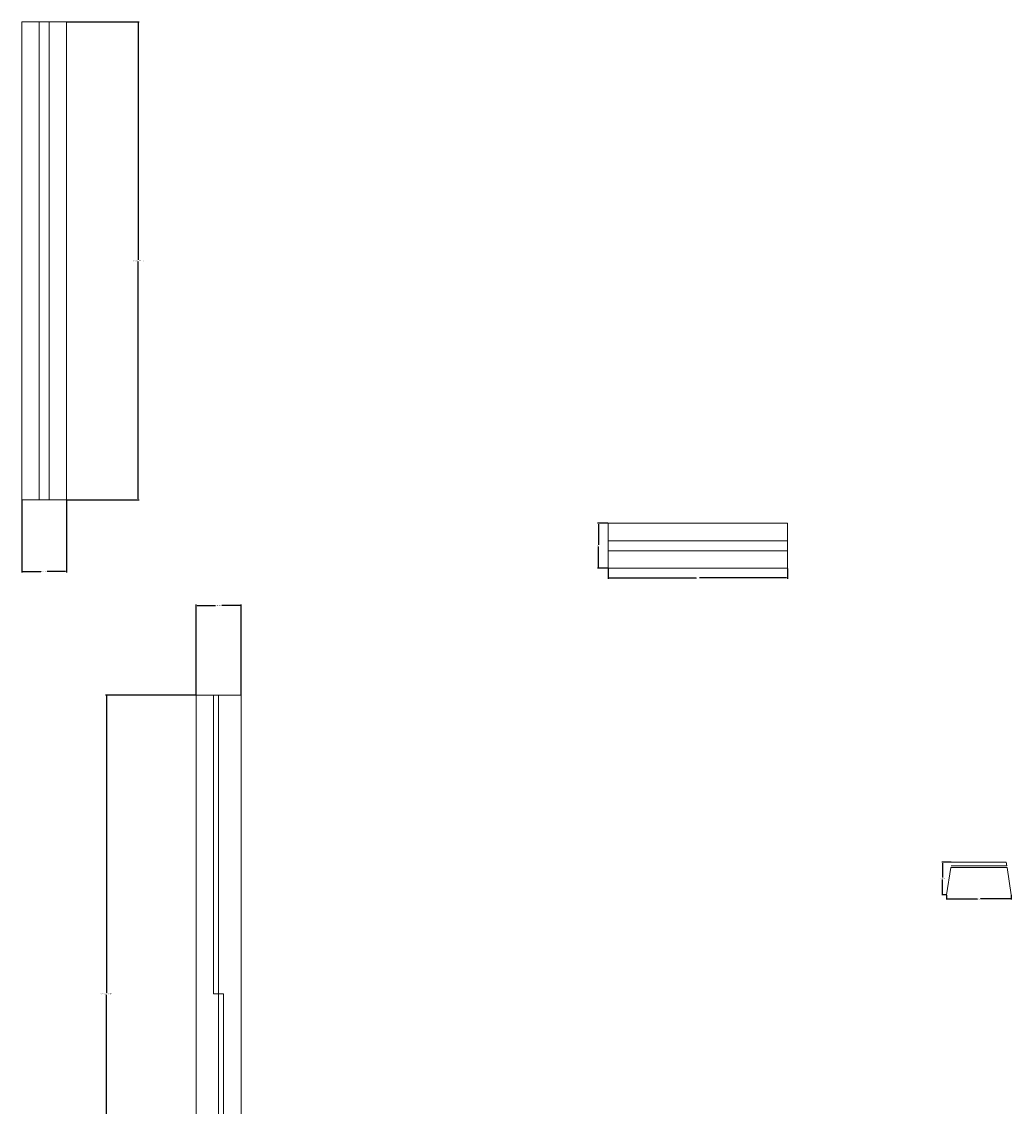
# Model space of a CAD drawing. Units: inches. Extents: x 226 to 1155, y 22 to 494.
# Tile 7 of 7: x 952 to 1150, y 276 to 494. Entities that reach past the tile are written whole.
import ezdxf

# ---------------------------------------------------------------- set-up
doc = ezdxf.new("R2010")
doc.units = ezdxf.units.IN
doc.header["$MEASUREMENT"] = 0
for name, color, linetype, lineweight in [('A-ANNO-DIMS', 2, 'Continuous', 18), ('A-FURN', 8, 'Continuous', 18), ('A-GLAZ', 4, 'Continuous', 18)]:
    doc.layers.add(name, color=color, linetype=linetype, lineweight=lineweight)
doc.styles.get("Standard").update_dxf_attribs({"font": 'arial.ttf'})
doc.dimstyles.get("Standard").update_dxf_attribs({"dimtxt": 0.18, "dimasz": 0.18, "dimexe": 0.18, "dimexo": 0.0625, "dimgap": 0.09, "dimtad": 0, "dimtih": 1, "dimtoh": 1, "dimdec": 4, "dimzin": 0, "dimdsep": 46, "dimlunit": 4, "dimtxsty": 'Standard', "dimcen": 0.09, "dimadec": 0, "dimazin": 0, "dimtfac": 1, "dimtdec": 4, "dimtofl": 0, "dimtmove": 0, "dimatfit": 3, "dimfxl": 1, "dimtolj": 1, "dimtzin": 0, "dimarcsym": 0})

# ---------------------------------------------------------------- blocks, each defined once
blk = doc.blocks.new('WIN-96')
for p, q in [((3.5, 96), (3.5, 0)), ((5.5, 96), (5.5, 0))]:
    blk.add_line(p, q)
blk.add_lwpolyline([(9, 96), (9, 0), (0, 0), (0, 96)], close=True)
blk = doc.blocks.new('WIN-120-SLIDING')
blk.add_lwpolyline([(9, 0), (0, 0), (0, 120), (9, 120)], close=True)
for points in [[(5.5, 0), (5.5, 60), (4.5, 60), (3.5, 60), (3.5, 120)], [(4.5, 0), (4.5, 60), (4.5, 120)]]:
    blk.add_lwpolyline(points)
blk = doc.blocks.new('*D42')
at = {"layer": 'A-ANNO-DIMS', "color": 0, "lineweight": -2, "transparency": 16777216}
for p, q in [((960.88, 493.93), (975.4, 493.93)), ((975.22, 493.75), (975.22, 446.12)), ((975.22, 398.11), (975.22, 445.75)), ((960.88, 397.93), (975.4, 397.93))]:
    blk.add_line(p, q, dxfattribs=at)
at = {"layer": 'A-ANNO-DIMS', "color": 0, "transparency": 16777216}
for points in [[(975.19, 493.75), (975.25, 493.75), (975.22, 493.93)], [(975.19, 398.11), (975.25, 398.11), (975.22, 397.93)]]:
    blk.add_solid(points, dxfattribs=at)
at = {"layer": 'Defpoints', "color": 0, "transparency": 16777216}
for p in [(960.82, 493.93), (975.22, 493.93), (960.82, 397.93)]:
    blk.add_point(p, dxfattribs=at)
at = {"layer": 'A-ANNO-DIMS', "color": 0, "transparency": 16777216, "insert": (975.22, 445.93), "char_height": 0.18, "attachment_point": 5}
blk.add_mtext('\\A1;WINDOW 8\'-0" TYP.', dxfattribs=at)
blk = doc.blocks.new('*D43')
at = {"layer": 'A-ANNO-DIMS', "color": 0, "lineweight": -2, "transparency": 16777216}
for p, q in [((951.82, 397.87), (951.82, 383.35)), ((960.82, 397.87), (960.82, 383.35)), ((952, 383.53), (955.68, 383.53)), ((960.64, 383.53), (956.96, 383.53))]:
    blk.add_line(p, q, dxfattribs=at)
at = {"layer": 'A-ANNO-DIMS', "color": 0, "transparency": 16777216}
for points in [[(952, 383.56), (952, 383.5), (951.82, 383.53)], [(960.64, 383.56), (960.64, 383.5), (960.82, 383.53)]]:
    blk.add_solid(points, dxfattribs=at)
at = {"layer": 'Defpoints', "color": 0, "transparency": 16777216}
for p in [(951.82, 397.93), (960.82, 397.93), (960.82, 383.53)]:
    blk.add_point(p, dxfattribs=at)
at = {"layer": 'A-ANNO-DIMS', "color": 0, "transparency": 16777216, "insert": (956.32, 383.53), "char_height": 0.18, "attachment_point": 5}
blk.add_mtext('\\A1;0\'-9" TYP.', dxfattribs=at)
blk = doc.blocks.new('*D44')
at = {"layer": 'A-ANNO-DIMS', "color": 0, "lineweight": -2, "transparency": 16777216}
for p, q in [((986.79, 358.71), (968.67, 358.71)), ((968.85, 358.53), (968.85, 298.89)), ((968.85, 238.89), (968.85, 298.53)), ((986.79, 238.71), (968.67, 238.71))]:
    blk.add_line(p, q, dxfattribs=at)
at = {"layer": 'A-ANNO-DIMS', "color": 0, "transparency": 16777216}
for points in [[(968.82, 358.53), (968.88, 358.53), (968.85, 358.71)], [(968.82, 238.89), (968.88, 238.89), (968.85, 238.71)]]:
    blk.add_solid(points, dxfattribs=at)
at = {"layer": 'Defpoints', "color": 0, "transparency": 16777216}
for p in [(968.85, 358.71), (986.85, 358.71), (986.85, 238.71)]:
    blk.add_point(p, dxfattribs=at)
at = {"layer": 'A-ANNO-DIMS', "color": 0, "transparency": 16777216, "insert": (968.85, 298.71), "char_height": 0.18, "attachment_point": 5}
blk.add_mtext('\\A1;WINDOW 10\'-0" TYP.', dxfattribs=at)
blk = doc.blocks.new('*D45')
at = {"layer": 'A-ANNO-DIMS', "color": 0, "lineweight": -2, "transparency": 16777216}
for p, q in [((986.85, 358.77), (986.85, 376.89)), ((995.85, 358.77), (995.85, 376.89)), ((987.03, 376.71), (990.71, 376.71)), ((995.67, 376.71), (991.99, 376.71))]:
    blk.add_line(p, q, dxfattribs=at)
at = {"layer": 'A-ANNO-DIMS', "color": 0, "transparency": 16777216}
for points in [[(987.03, 376.74), (987.03, 376.68), (986.85, 376.71)], [(995.67, 376.74), (995.67, 376.68), (995.85, 376.71)]]:
    blk.add_solid(points, dxfattribs=at)
at = {"layer": 'Defpoints', "color": 0, "transparency": 16777216}
for p in [(995.85, 376.71), (986.85, 358.71), (995.85, 358.71)]:
    blk.add_point(p, dxfattribs=at)
at = {"layer": 'A-ANNO-DIMS', "color": 0, "transparency": 16777216, "insert": (991.35, 376.71), "char_height": 0.18, "attachment_point": 5}
blk.add_mtext('\\A1;0\'-9" TYP.', dxfattribs=at)
blk = doc.blocks.new('*D91')
at = {"layer": 'A-ANNO-DIMS', "color": 0, "lineweight": -2, "transparency": 16777216}
for p, q in [((1069.54, 384.15), (1069.54, 382.08)), ((1105.54, 384.15), (1105.54, 382.08)), ((1069.72, 382.26), (1087.21, 382.26)), ((1105.36, 382.26), (1087.87, 382.26))]:
    blk.add_line(p, q, dxfattribs=at)
at = {"layer": 'A-ANNO-DIMS', "color": 0, "transparency": 16777216}
for points in [[(1069.72, 382.29), (1069.72, 382.23), (1069.54, 382.26)], [(1105.36, 382.29), (1105.36, 382.23), (1105.54, 382.26)]]:
    blk.add_solid(points, dxfattribs=at)
at = {"layer": 'Defpoints', "color": 0, "transparency": 16777216}
for p in [(1069.54, 384.21), (1105.54, 384.21), (1105.54, 382.26)]:
    blk.add_point(p, dxfattribs=at)
at = {"layer": 'A-ANNO-DIMS', "color": 0, "transparency": 16777216, "insert": (1087.54, 382.26), "char_height": 0.18, "attachment_point": 5}
blk.add_mtext('\\A1;3\'-0"', dxfattribs=at)
blk = doc.blocks.new('*D92')
at = {"layer": 'A-ANNO-DIMS', "color": 0, "lineweight": -2, "transparency": 16777216}
for p, q in [((1069.47, 393.21), (1067.41, 393.21)), ((1067.59, 393.03), (1067.59, 388.89)), ((1067.59, 384.39), (1067.59, 388.53)), ((1069.47, 384.21), (1067.41, 384.21))]:
    blk.add_line(p, q, dxfattribs=at)
at = {"layer": 'A-ANNO-DIMS', "color": 0, "transparency": 16777216}
for points in [[(1067.56, 393.03), (1067.62, 393.03), (1067.59, 393.21)], [(1067.56, 384.39), (1067.62, 384.39), (1067.59, 384.21)]]:
    blk.add_solid(points, dxfattribs=at)
at = {"layer": 'Defpoints', "color": 0, "transparency": 16777216}
for p in [(1067.59, 393.21), (1069.54, 393.21), (1069.54, 384.21)]:
    blk.add_point(p, dxfattribs=at)
at = {"layer": 'A-ANNO-DIMS', "color": 0, "transparency": 16777216, "insert": (1067.59, 388.71), "char_height": 0.18, "attachment_point": 5}
blk.add_mtext('\\A1;0\'-9"', dxfattribs=at)
blk = doc.blocks.new('*D93')
at = {"layer": 'A-ANNO-DIMS', "color": 0, "lineweight": -2, "transparency": 16777216}
for p, q in [((1137.49, 318.56), (1137.49, 317.64)), ((1150.48, 318.56), (1150.48, 317.64)), ((1137.67, 317.82), (1143.67, 317.82)), ((1150.3, 317.82), (1144.31, 317.82))]:
    blk.add_line(p, q, dxfattribs=at)
at = {"layer": 'A-ANNO-DIMS', "color": 0, "transparency": 16777216}
for points in [[(1137.67, 317.85), (1137.67, 317.79), (1137.49, 317.82)], [(1150.3, 317.85), (1150.3, 317.79), (1150.48, 317.82)]]:
    blk.add_solid(points, dxfattribs=at)
at = {"layer": 'Defpoints', "color": 0, "transparency": 16777216}
for p in [(1137.49, 318.62), (1150.48, 318.62), (1150.48, 317.82)]:
    blk.add_point(p, dxfattribs=at)
at = {"layer": 'A-ANNO-DIMS', "color": 0, "transparency": 16777216, "insert": (1143.99, 317.82), "char_height": 0.18, "attachment_point": 5}
blk.add_mtext('\\A1;1\'-1"', dxfattribs=at)
blk = doc.blocks.new('*D94')
at = {"layer": 'A-ANNO-DIMS', "color": 0, "lineweight": -2, "transparency": 16777216}
for p, q in [((1138.44, 325.13), (1136.51, 325.13)), ((1136.69, 324.95), (1136.69, 322.06)), ((1136.69, 318.8), (1136.69, 321.69)), ((1137.43, 318.62), (1136.51, 318.62))]:
    blk.add_line(p, q, dxfattribs=at)
at = {"layer": 'A-ANNO-DIMS', "color": 0, "transparency": 16777216}
for points in [[(1136.66, 324.95), (1136.72, 324.95), (1136.69, 325.13)], [(1136.66, 318.8), (1136.72, 318.8), (1136.69, 318.62)]]:
    blk.add_solid(points, dxfattribs=at)
at = {"layer": 'Defpoints', "color": 0, "transparency": 16777216}
for p in [(1136.69, 325.13), (1138.51, 325.13), (1137.49, 318.62)]:
    blk.add_point(p, dxfattribs=at)
at = {"layer": 'A-ANNO-DIMS', "color": 0, "transparency": 16777216, "insert": (1136.69, 321.87), "char_height": 0.18, "attachment_point": 5}
blk.add_mtext('\\A1;0\'-6 1/2"', dxfattribs=at)

msp = doc.modelspace()

# ---------------------------------------------------------------- linework, layer by layer
at = {"layer": 'A-FURN'}
for p, q in [((1138.50647, 325.12906), (1149.46566, 325.12906)), ((1149.57272, 324.44388), (1149.46566, 325.12906)), ((1138.34599, 324.10204), (1137.48953, 318.62041)), ((1138.34866, 324.10163), (1149.6295, 324.10163)), ((1149.57416, 324.44411), (1138.4014, 324.44411)), ((1150.48268, 318.62041), (1149.62629, 324.10113))]:
    msp.add_line(p, q, dxfattribs=at)
at = {"layer": 'A-GLAZ'}
for p, q in [((1069.53684, 393.21), (1105.53684, 393.21)), ((1069.53684, 384.21), (1069.53684, 393.21)), ((1105.53684, 393.21), (1105.53684, 384.21)), ((1069.53684, 389.71), (1105.53684, 389.71)), ((1069.53684, 387.71), (1105.53684, 387.71)), ((1105.53684, 384.21), (1069.53684, 384.21))]:
    msp.add_line(p, q, dxfattribs=at)

# ---------------------------------------------------------------- block references
for name, p in [('WIN-96', (951.82198, 397.93229)), ('WIN-120-SLIDING', (986.85159, 238.70877))]:
    msp.add_blockref(name, p, dxfattribs=at)

# ---------------------------------------------------------------- dimensions: what is measured, and where the dimension line sits
at = {"layer": 'A-ANNO-DIMS'}
for base, p1, p2, picture, middle in [((975.22183, 493.93194), (960.82183, 397.93194), (960.82183, 493.93194), '*D42', (975.22183, 445.93194)), ((968.85144, 358.70847), (986.85144, 238.70847), (986.85144, 358.70847), '*D44', (968.85144, 298.70847))]:
    dim = msp.add_linear_dim(base=base, p1=p1, p2=p2, angle=90, text='WINDOW <> TYP.', dimstyle='Standard', override={"dimdec": 1, "dimlfac": 1, "dimrnd": 0, "dimzin": 1, "dimdsep": 46, "dimlunit": 4, "dimfrac": 2}, dxfattribs=at)
    dim.commit()
    dim.dimension.update_dxf_attribs({"geometry": picture, "text_midpoint": middle})
for base, p1, p2, picture, middle in [((960.82183, 383.53194), (951.82183, 397.93194), (960.82183, 397.93194), '*D43', (956.32183, 383.53194)), ((995.85144, 376.70847), (986.85144, 358.70847), (995.85144, 358.70847), '*D45', (991.35144, 376.70847))]:
    dim = msp.add_linear_dim(base=base, p1=p1, p2=p2, text='<> TYP.', dimstyle='Standard', override={"dimdec": 1, "dimlfac": 1, "dimrnd": 0, "dimzin": 1, "dimdsep": 46, "dimlunit": 4, "dimfrac": 2}, dxfattribs=at)
    dim.commit()
    dim.dimension.update_dxf_attribs({"geometry": picture, "text_midpoint": middle})
for base, p1, p2, picture, middle in [((1067.58684, 393.21), (1069.53684, 384.21), (1069.53684, 393.21), '*D92', (1067.58684, 388.71)), ((1136.68953, 325.12906), (1137.48953, 318.62041), (1138.50647, 325.12906), '*D94', (1136.68953, 321.87473))]:
    dim = msp.add_linear_dim(base=base, p1=p1, p2=p2, angle=90, dimstyle='Standard', override={"dimdec": 1, "dimlfac": 1, "dimrnd": 0, "dimzin": 1, "dimdsep": 46, "dimlunit": 4, "dimfrac": 2}, dxfattribs=at)
    dim.commit()
    dim.dimension.update_dxf_attribs({"geometry": picture, "text_midpoint": middle})
for base, p1, p2, picture, middle in [((1105.53684, 382.26), (1069.53684, 384.21), (1105.53684, 384.21), '*D91', (1087.53684, 382.26)), ((1150.48268, 317.82041), (1137.48953, 318.62041), (1150.48268, 318.62041), '*D93', (1143.9861, 317.82041))]:
    dim = msp.add_linear_dim(base=base, p1=p1, p2=p2, dimstyle='Standard', override={"dimdec": 1, "dimlfac": 1, "dimrnd": 0, "dimzin": 1, "dimdsep": 46, "dimlunit": 4, "dimfrac": 2}, dxfattribs=at)
    dim.commit()
    dim.dimension.update_dxf_attribs({"geometry": picture, "text_midpoint": middle})

doc.saveas('drawing.dxf')
